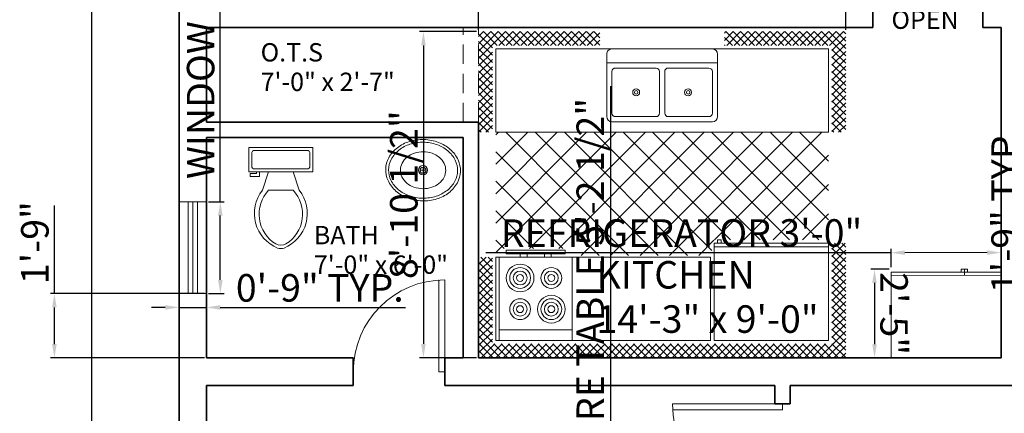
# Model space of a CAD drawing. Units: inches. Extents: x 1885 to 4781, y 1153 to 4395.
# Tile 2 of 7: x 2309 to 2631, y 1657 to 1786. Entities that reach past the tile are written whole.
import ezdxf

# ---------------------------------------------------------------- set-up
doc = ezdxf.new("R2010")
doc.units = ezdxf.units.IN
doc.linetypes.add('HIDDEN', pattern=[9.525, 6.35, -3.175])
doc.layers.add('A-ANNO-DIMS', color=5, linetype='Continuous', lineweight=18)
doc.layers.add('A-WALL', color=7, linetype='Continuous', lineweight=35)
for name, color, linetype, lineweight, true_color in [('A-ANNO-TEXT', 244, 'Continuous', 18, 0x991b1e), ('A-AREA-IDEN', 244, 'Continuous', 18, 0x991b1e), ('A-DOOR', 11, 'Continuous', 18, 0xf27172), ('A-EQPM', 11, 'Continuous', 18, 0xf27172), ('A-FLOR-FIXT', 11, 'Continuous', 18, 0xf27172), ('A-GLAZ', 152, 'Continuous', 18, 0x2776bb), ('A-WALL-HIDN', 11, 'HIDDEN', 18, 0xf27172)]:
    doc.layers.add(name, color=color, linetype=linetype, lineweight=lineweight, true_color=true_color)
doc.styles.get("Standard").update_dxf_attribs({"font": 'arial.ttf'})
doc.dimstyles.new('ISO-25', dxfattribs={"dimtxt": 9, "dimasz": 4.5, "dimexe": 1.25, "dimexo": 0.625, "dimtad": 1, "dimdec": 0, "dimlunit": 3, "dimtxsty": 'Standard', "dimcen": 2.5, "dimadec": 0, "dimazin": 0, "dimtfac": 1, "dimtdec": 0, "dimtmove": 0, "dimatfit": 3, "dimfxl": 1, "dimarcsym": 0})

# ---------------------------------------------------------------- blocks, each defined once
blk = doc.blocks.new('Kitchen Layout - 7 x 8 ft')
for p, q in [((-5, 81.32), (2.68, 89)), ((-5, 83.44), (0.56, 89)), ((-5, 85.56), (-1.56, 89)), ((-5, 87.68), (-3.68, 89)), ((-1, 84.97), (-5, 88.97)), ((1.09, 85), (-2.91, 89)), ((3.21, 85), (-0.79, 89)), ((0.81, 85), (4.81, 89)), ((5.34, 85), (1.34, 89)), ((2.93, 85), (6.93, 89)), ((7.46, 85), (3.46, 89)), ((5.05, 85), (9.05, 89)), ((9.58, 85), (5.58, 89)), ((7.17, 85), (11.17, 89)), ((11.7, 85), (7.7, 89)), ((9.29, 85), (13.29, 89)), ((13.82, 85), (9.82, 89)), ((11.41, 85), (15.41, 89)), ((15.94, 85), (11.94, 89)), ((13.53, 85), (17.53, 89)), ((18.06, 85), (14.06, 89)), ((15.65, 85), (19.65, 89)), ((20.18, 85), (16.18, 89)), ((17.78, 85), (21.78, 89)), ((22.31, 85), (18.31, 89)), ((19.9, 85), (23.9, 89)), ((24.43, 85), (20.43, 89)), ((22.02, 85), (26.02, 89)), ((26.55, 85), (22.55, 89)), ((24.14, 85), (28.14, 89)), ((28.67, 85), (24.67, 89)), ((26.26, 85), (30.26, 89)), ((30.79, 85), (26.79, 89)), ((28.38, 85), (32.38, 89)), ((32.91, 85), (28.91, 89)), ((30.5, 85), (34.5, 89)), ((35.03, 85), (31.03, 89)), ((32.63, 85), (36.63, 89)), ((37.16, 85), (33.16, 89)), ((34.75, 85), (38.75, 89)), ((39.28, 85), (35.28, 89)), ((36.87, 85), (40.87, 89)), ((41.4, 85), (37.4, 89)), ((38.99, 85), (42.99, 89)), ((43.52, 85), (39.52, 89)), ((41.11, 85), (45.11, 89)), ((45.64, 85), (41.64, 89)), ((43.23, 85), (47.23, 89)), ((47.76, 85), (43.76, 89)), ((45.35, 85), (49.35, 89)), ((49.88, 85), (45.88, 89)), ((47.47, 85), (51.47, 89)), ((52, 85), (48, 89)), ((49.6, 85), (53.6, 89)), ((54.13, 85), (50.13, 89)), ((51.72, 85), (55.72, 89)), ((56.25, 85), (52.25, 89)), ((53.84, 85), (57.84, 89)), ((58.37, 85), (54.37, 89)), ((55.96, 85), (59.96, 89)), ((60.49, 85), (56.49, 89)), ((58.08, 85), (62.08, 89)), ((62.61, 85), (58.61, 89)), ((60.2, 85), (64.2, 89)), ((64.73, 85), (60.73, 89)), ((62.32, 85), (66.32, 89)), ((66.85, 85), (62.85, 89)), ((64.45, 85), (68.45, 89)), ((68.97, 85), (64.97, 89)), ((66.57, 85), (70.57, 89)), ((71.1, 85), (67.1, 89)), ((68.69, 85), (72.69, 89)), ((73.22, 85), (69.22, 89)), ((70.81, 85), (74.81, 89)), ((75.34, 85), (71.34, 89)), ((72.93, 85), (76.93, 89)), ((77.46, 85), (73.46, 89)), ((75.05, 85), (79.05, 89)), ((79.58, 85), (75.58, 89)), ((77.17, 85), (81.17, 89)), ((81.7, 85), (77.7, 89)), ((79.29, 85), (83.29, 89)), ((83.82, 85), (79.82, 89)), ((81.42, 85), (85.42, 89)), ((85.95, 85), (81.95, 89)), ((83.54, 85), (87.54, 89)), ((88.07, 85), (84.07, 89)), ((85.66, 85), (89.66, 89)), ((90.19, 85), (86.19, 89)), ((87.78, 85), (91.78, 89)), ((92.31, 85), (88.31, 89)), ((89.9, 85), (93.9, 89)), ((94.43, 85), (90.43, 89)), ((92.02, 85), (96.02, 89)), ((96.55, 85), (92.55, 89)), ((94.14, 85), (98.14, 89)), ((101, 82.67), (94.67, 89)), ((96.27, 85), (100.27, 89)), ((101, 84.79), (96.79, 89)), ((101, 86.92), (98.92, 89)), ((-1, 82.85), (-5, 86.85)), ((97, 83.61), (101, 87.61)), ((97, 81.49), (101, 85.49)), ((-1, 80.73), (-5, 84.73)), ((-5, 79.19), (-1, 83.19)), ((-1, 78.61), (-5, 82.61)), ((34, 84), (96, 84)), ((34, 60), (34, 84)), ((96, 84), (96, 60)), ((101, 80.55), (97, 84.55)), ((97, 79.37), (101, 83.37)), ((-5, 77.07), (-1, 81.07)), ((-1, 76.49), (-5, 80.49)), ((74, 81), (95, 81)), ((101, 78.43), (97, 82.43)), ((97, 77.25), (101, 81.25)), ((101, 76.31), (97, 80.31)), ((-5, 74.95), (-1, 78.95)), ((-1, 74.36), (-5, 78.36)), ((-5, 72.83), (-1, 76.83)), ((97, 75.13), (101, 79.13)), ((101, 74.19), (97, 78.19)), ((97, 73.01), (101, 77.01)), ((-1, 72.24), (-5, 76.24)), ((-5, 70.71), (-1, 74.71)), ((-1, 70.12), (-5, 74.12)), ((101, 72.07), (97, 76.07)), ((97, 70.89), (101, 74.89)), ((101, 69.95), (97, 73.95)), ((-5, 68.59), (-1, 72.59)), ((-1, 68), (-5, 72)), ((97, 68.76), (101, 72.76)), ((101, 67.82), (97, 71.82)), ((-5, 66.47), (-1, 70.47)), ((-1, 65.88), (-5, 69.88)), ((-5, 64.35), (-1, 68.35)), ((97, 66.64), (101, 70.64)), ((101, 65.7), (97, 69.7)), ((97, 64.52), (101, 68.52)), ((-1, 63.76), (-5, 67.76)), ((-5, 62.22), (-1, 66.22)), ((-1, 61.64), (-5, 65.64)), ((101, 63.58), (97, 67.58)), ((97, 62.4), (101, 66.4)), ((101, 61.46), (97, 65.46)), ((-5, 60.1), (-1, 64.1)), ((-1, 59.52), (-5, 63.52)), ((97, 60.28), (101, 64.28)), ((100.34, 60), (97, 63.34)), ((-5, 57.98), (-1, 61.98)), ((-1, 57.39), (-5, 61.39)), ((-4.86, 56), (-1, 59.86)), ((96, 60), (34, 60)), ((80, 60), (80, 59)), ((82, 59), (82, 60)), ((87, 59), (87, 60)), ((89, 60), (89, 59)), ((98.22, 60), (97, 61.22)), ((98.84, 60), (101, 62.16)), ((100.96, 60), (101, 60.04)), ((-1.73, 56), (-5, 59.27)), ((-3.85, 56), (-5, 57.15)), ((-2.74, 56), (-1, 57.74)), ((0, 57), (33, 57)), ((10.4, 24), (45.9, 59.5)), ((18.88, 24), (54.38, 59.5)), ((27.37, 24), (62.87, 59.5)), ((33.03, 55.11), (37.41, 59.5)), ((67.71, 24), (33.68, 58.04)), ((35.85, 24), (71.35, 59.5)), ((76.2, 24), (40.7, 59.5)), ((44.34, 24), (77.84, 57.5)), ((84.68, 24), (49.18, 59.5)), ((52.82, 24), (86.32, 57.5)), ((93.17, 24), (57.67, 59.5)), ((61.31, 24), (96, 58.69)), ((96, 29.65), (66.15, 59.5)), ((96, 38.14), (76.64, 57.5)), ((96, 46.63), (85.13, 57.5)), ((96, 55.11), (93.57, 57.54)), ((0, 30.57), (24.43, 55)), ((0, 39.06), (15.94, 55)), ((0, 47.54), (7.46, 55)), ((1.91, 24), (32.91, 55)), ((33.77, 24), (2.77, 55)), ((42.26, 24), (11.26, 55)), ((50.74, 24), (19.74, 55)), ((59.23, 24), (28.23, 55)), ((31, 55), (31, 56)), ((32, 55), (31, 55)), ((32, 56), (32, 55)), ((25.29, 24), (0, 49.29)), ((69.79, 24), (96, 50.21)), ((16.8, 24), (0, 40.8)), ((78.28, 24), (96, 41.72)), ((8.32, 24), (0, 32.32)), ((86.76, 24), (96, 33.24)), ((-5, 21.92), (-2.92, 24)), ((-5, 19.8), (-1, 23.8)), ((-1, 19.21), (-5, 23.21)), ((-1, 21.33), (-3.67, 24)), ((-1, 23.45), (-1.55, 24)), ((0, 24), (96, 24)), ((0, 0), (0, 24)), ((95.25, 24), (96, 24.75)), ((96, 24), (96, 0)), ((97, 22.1), (98.9, 24)), ((97, 19.97), (101, 23.97)), ((101, 19.03), (97, 23.03)), ((101, 21.16), (98.16, 24)), ((101, 23.28), (100.28, 24)), ((-5, 17.68), (-1, 21.68)), ((-1, 17.09), (-5, 21.09)), ((97, 17.85), (101, 21.85)), ((101, 16.91), (97, 20.91)), ((-5, 15.55), (-1, 19.55)), ((-1, 14.97), (-5, 18.97)), ((-5, 13.43), (-1, 17.43)), ((47.25, 6.5), (47.25, 18.5)), ((48.75, 18.5), (48.75, 6.5)), ((97, 15.73), (101, 19.73)), ((101, 14.79), (97, 18.79)), ((97, 13.61), (101, 17.61)), ((-1, 12.85), (-5, 16.85)), ((-5, 11.31), (-1, 15.31)), ((-1, 10.73), (-5, 14.73)), ((101, 12.67), (97, 16.67)), ((97, 11.49), (101, 15.49)), ((101, 10.55), (97, 14.55)), ((-5, 9.19), (-1, 13.19)), ((-1, 8.6), (-5, 12.6)), ((97, 9.37), (101, 13.37)), ((101, 8.43), (97, 12.43)), ((-5, 7.07), (-1, 11.07)), ((-1, 6.48), (-5, 10.48)), ((-5, 4.95), (-1, 8.95)), ((97, 7.25), (101, 11.25)), ((101, 6.31), (97, 10.31)), ((97, 5.12), (101, 9.12)), ((-1, 4.36), (-5, 8.36)), ((-5, 2.83), (-1, 6.83)), ((-1, 2.24), (-5, 6.24)), ((101, 4.18), (97, 8.18)), ((97, 3), (101, 7)), ((101, 2.06), (97, 6.06)), ((-5, 0.71), (-1, 4.71)), ((-1, 0.12), (-5, 4.12)), ((64, 4), (32, 4)), ((97, 0.88), (101, 4.88)), ((101, -0.06), (97, 3.94)), ((-5, -1.42), (-1, 2.58)), ((2, -5), (-5, 2)), ((-5, -3.54), (-1, 0.46)), ((96, 0), (0, 0)), ((93.24, -5), (101, 2.76)), ((95.36, -5), (101, 0.64)), ((101, -2.18), (97, 1.82)), ((-0.12, -5), (-5, -0.12)), ((-2.25, -5), (-5, -2.25)), ((-4.34, -5), (-0.34, -1)), ((-2.22, -5), (1.78, -1)), ((-0.1, -5), (3.9, -1)), ((4.12, -5), (0.12, -1)), ((2.02, -5), (6.02, -1)), ((6.24, -5), (2.24, -1)), ((4.14, -5), (8.14, -1)), ((8.36, -5), (4.36, -1)), ((6.27, -5), (10.27, -1)), ((10.48, -5), (6.48, -1)), ((8.39, -5), (12.39, -1)), ((12.6, -5), (8.6, -1)), ((10.51, -5), (14.51, -1)), ((14.73, -5), (10.73, -1)), ((12.63, -5), (16.63, -1)), ((16.85, -5), (12.85, -1)), ((14.75, -5), (18.75, -1)), ((18.97, -5), (14.97, -1)), ((16.87, -5), (20.87, -1)), ((21.09, -5), (17.09, -1)), ((18.99, -5), (22.99, -1)), ((23.21, -5), (19.21, -1)), ((21.11, -5), (25.11, -1)), ((25.33, -5), (21.33, -1)), ((23.24, -5), (27.24, -1)), ((27.45, -5), (23.45, -1)), ((25.36, -5), (29.36, -1)), ((29.57, -5), (25.57, -1)), ((27.48, -5), (30, -2.48)), ((30, -3.3), (27.7, -1)), ((30, -1.18), (29.82, -1)), ((66, -2.54), (67.54, -1)), ((66, -4.66), (69.66, -1)), ((69.88, -5), (66, -1.12)), ((67.78, -5), (71.78, -1)), ((72, -5), (68, -1)), ((69.9, -5), (73.9, -1)), ((74.12, -5), (70.12, -1)), ((72.03, -5), (76.03, -1)), ((76.24, -5), (72.24, -1)), ((74.15, -5), (78.15, -1)), ((78.36, -5), (74.36, -1)), ((76.27, -5), (80.27, -1)), ((80.49, -5), (76.49, -1)), ((78.39, -5), (82.39, -1)), ((82.61, -5), (78.61, -1)), ((80.51, -5), (84.51, -1)), ((84.73, -5), (80.73, -1)), ((82.63, -5), (86.63, -1)), ((86.85, -5), (82.85, -1)), ((84.75, -5), (88.75, -1)), ((88.97, -5), (84.97, -1)), ((86.88, -5), (90.88, -1)), ((91.09, -5), (87.09, -1)), ((89, -5), (93, -1)), ((93.21, -5), (89.21, -1)), ((91.12, -5), (95.12, -1)), ((95.34, -5), (91.34, -1)), ((97.46, -5), (93.46, -1)), ((99.58, -5), (95.58, -1)), ((101, -4.3), (97, -0.3)), ((97.48, -5), (101, -1.48)), ((-4.37, -5), (-5, -4.37)), ((29.6, -5), (30, -4.6)), ((67.76, -5), (66, -3.24)), ((99.6, -5), (101, -3.6))]:
    blk.add_line(p, q)
for points in [[(0, 56), (0, 84), (33, 84), (33, 56)], [(74, 60), (74, 84), (95, 84), (95, 60)], [(76, 58), (76, 59), (93, 59), (93, 58)]]:
    blk.add_lwpolyline(points, close=True)
for points in [[(33.5, 21), (62.5, 21)], [(32, 1.5), (32, 19.5)], [(33.5, 6.5), (33.5, 18.5)], [(34.5, 19.5), (46.25, 19.5)], [(49.75, 19.5), (61.5, 19.5)], [(62.5, 18.5), (62.5, 6.5)], [(64, 19.5), (64, 1.5)], [(46.25, 5.5), (34.5, 5.5)], [(61.5, 5.5), (49.75, 5.5)], [(62.5, 0), (33.5, 0)]]:
    blk.add_lwpolyline(points)
for centre, radius in [((80, 75), 4), ((80, 75), 3), ((80, 75), 2), ((89, 75), 3), ((89, 75), 2), ((80, 75), 1), ((89, 75), 1), ((80, 66), 3), ((89, 66), 4), ((89, 66), 3), ((80, 66), 2), ((80, 66), 1), ((89, 66), 2), ((89, 66), 1), ((40.5, 12.5), 1), ((40.5, 12.5), 0.5), ((55.5, 12.5), 1), ((55.5, 12.5), 0.5)]:
    blk.add_circle(centre, radius)
for centre, radius, start, end in [((33.5, 19.5), 1.5, 90, 180), ((62.5, 19.5), 1.5, 0, 90), ((34.5, 18.5), 1, 90, 180), ((46.25, 18.5), 1, 0, 90), ((49.75, 18.5), 1, 90, 180), ((61.5, 18.5), 1, 0, 90), ((34.5, 6.5), 1, 180, 270), ((46.25, 6.5), 1, 270, 0), ((49.75, 6.5), 1, 180, 270), ((61.5, 6.5), 1, 270, 0), ((33.5, 1.5), 1.5, 180, 270), ((62.5, 1.5), 1.5, 270, 0)]:
    blk.add_arc(centre, radius, start, end)
blk = doc.blocks.new('Refrigerator-2 door - 36 in top')
for p, q in [((0, -26.999999), (36, -26.999999)), ((11, -27.999999), (11, -28.999999)), ((12, -26.999999), (12, -28.999999)), ((13, -28.999999), (13, -27.999999)), ((11, -28.999999), (13, -28.999999))]:
    blk.add_line(p, q)
blk.add_lwpolyline([(0, -27.999999), (0, 0), (36, 0), (36, -27.999999)], close=True)
blk = doc.blocks.new('Toilet - top')
for p, q in [((9.5, -6), (9.5, -2)), ((-10, -8.5), (-8, -8.5)), ((-10, -9.5), (-10, -8.5)), ((-7, -9.5), (-10, -9.5)), ((-8, -8.5), (-8, -8)), ((-7, -8), (-7, -9.5)), ((-4, -8), (-6, -14)), ((4, -8), (6, -14)), ((4, -14), (-4, -14))]:
    blk.add_line(p, q)
blk.add_lwpolyline([(10.5, -8), (10.5, 0), (-10.5, 0), (-10.5, -8)], close=True)
for points in [[(-9.5, -2), (-9.5, -6)], [(8.5, -1), (-8.5, -1)], [(-8.5, -7), (8.5, -7)]]:
    blk.add_lwpolyline(points)
for centre, radius, start, end in [((-8.62, -1.88), 0.884, 81.8699, 188.1301), ((8.62, -1.88), 0.884, 351.8699, 98.1301), ((-8.62, -6.12), 0.884, 171.8699, 278.1301), ((8.62, -6.12), 0.884, 261.8699, 8.1301), ((3.52, -21.58), 12.17, 141.4691, 247.9714), ((4.2, -21.82), 11.33, 136.3677, 238.9468), ((-3.52, -21.58), 12.17, 292.0284, 38.5307), ((-4.2, -21.82), 11.33, 301.053, 43.6321), ((0, -27.88), 4, 245.7318, 294.2682), ((0, -29), 4, 254.8605, 285.1395)]:
    blk.add_arc(centre, radius, start, end)
blk = doc.blocks.new('Sink - Oval top')
for p, q in [((-1, 0), (1, 0)), ((0, 1), (0, -1))]:
    blk.add_line(p, q)
for points in [[(-12.23, 0.39, 0.117634), (-11.46, -3.36, 0.104469), (-8.88, -6.8, 0.090016), (-5.08, -9.07, 0.08192), (-0.32, -10.02, 0.08192), (4.49, -9.38, 0.090016), (8.42, -7.36, 0.104469), (11.22, -4.09, 0.117634), (12.23, -0.39, 0.117634), (11.46, 3.36, 0.104469), (8.88, 6.8, 0.090016), (5.08, 9.07, 0.08192), (0.32, 10.02, 0.08192), (-4.49, 9.38, 0.090016), (-8.42, 7.36, 0.104469), (-11.22, 4.09, 0.117634)], [(-11.29, 0.16, 0.118622), (-10.52, -3.25, 0.104678), (-8.07, -6.36, 0.089562), (-4.54, -8.37, 0.081185), (-0.13, -9.15, 0.081185), (4.3, -8.49, 0.089562), (7.89, -6.58, 0.104678), (10.42, -3.55, 0.118622), (11.29, -0.16, 0.118622), (10.52, 3.25, 0.104678), (8.07, 6.36, 0.089562), (4.54, 8.37, 0.081185), (0.13, 9.15, 0.081185), (-4.3, 8.49, 0.089562), (-7.89, 6.58, 0.104678), (-10.42, 3.55, 0.118622)], [(-7.42, 0.08, 0.118283), (-6.91, -2.17, 0.104607), (-5.29, -4.21, 0.089718), (-2.97, -5.53, 0.081436), (-0.07, -6.04, 0.081436), (2.84, -5.59, 0.089718), (5.2, -4.33, 0.104607), (6.86, -2.32, 0.118283), (7.42, -0.08, 0.118283), (6.91, 2.17, 0.104607), (5.29, 4.21, 0.089718), (2.97, 5.53, 0.081436), (0.07, 6.04, 0.081436), (-2.84, 5.59, 0.089718), (-5.2, 4.33, 0.104607), (-6.86, 2.32, 0.118283)]]:
    blk.add_lwpolyline(points, format="xyb", close=True)
for radius in [1.5, 1]:
    blk.add_circle((0, 0), radius)
blk = doc.blocks.new('*D26')
at = {"layer": 'A-ANNO-DIMS', "color": 0, "lineweight": -2, "transparency": 16777216}
for p, q in [((2360.28, 2222.42), (2331.02, 2222.42)), ((2332.27, 2217.92), (2332.27, 1493.92)), ((2360.28, 1489.42), (2331.02, 1489.42))]:
    blk.add_line(p, q, dxfattribs=at)
at = {"layer": 'A-ANNO-DIMS', "color": 0, "transparency": 16777216}
for points in [[(2331.52, 2217.92), (2333.02, 2217.92), (2332.27, 2222.42)], [(2331.52, 1493.92), (2333.02, 1493.92), (2332.27, 1489.42)]]:
    blk.add_solid(points, dxfattribs=at)
at = {"layer": 'Defpoints', "color": 0, "transparency": 16777216}
for p in [(2360.91, 2222.42), (2332.27, 1489.42), (2360.91, 1489.42)]:
    blk.add_point(p, dxfattribs=at)
at = {"layer": 'A-ANNO-DIMS', "color": 0, "transparency": 16777216, "insert": (2327.04, 1855.92), "char_height": 9, "attachment_point": 5, "rotation": 90}
blk.add_mtext('61\'-1"', dxfattribs=at)
blk = doc.blocks.new('WIN-30IN')
for p, q in [((0, 0), (0, 30)), ((0, 30), (9, 30)), ((3, 0), (3, 30)), ((4.5, 0), (4.5, 30)), ((6, 0), (6, 30)), ((9, 30), (9, 0)), ((9, 0), (0, 0))]:
    blk.add_line(p, q)
blk = doc.blocks.new('DOOR-SWING-30IN')
for p, q in [((0, 2), (30, 2)), ((30, 0), (30, 2)), ((0, 0), (30, 0))]:
    blk.add_line(p, q)
blk.add_arc((30, 0), 30, 90, 180)
blk = doc.blocks.new('DOOR-SWING-36IN')
for p, q in [((0, 36), (0, 0)), ((2, 36), (2, 0)), ((0, 0), (2, 0))]:
    blk.add_line(p, q)
blk.add_arc((0, 0), 36, 0, 90)
blk = doc.blocks.new('*D47')
at = {"layer": 'A-ANNO-DIMS', "color": 0, "lineweight": -2, "transparency": 16777216}
for p, q in [((2374.41, 1726.42), (2374.41, 1846.06)), ((2370.53, 1726.42), (2375.66, 1726.42)), ((2374.41, 1700.92), (2374.41, 1721.92)), ((2370.53, 1696.42), (2375.66, 1696.42))]:
    blk.add_line(p, q, dxfattribs=at)
at = {"layer": 'A-ANNO-DIMS', "color": 0, "transparency": 16777216}
for points in [[(2373.66, 1721.92), (2375.16, 1721.92), (2374.41, 1726.42)], [(2373.66, 1700.92), (2375.16, 1700.92), (2374.41, 1696.42)]]:
    blk.add_solid(points, dxfattribs=at)
at = {"layer": 'Defpoints', "color": 0, "transparency": 16777216}
for p in [(2369.91, 1726.42), (2374.41, 1726.42), (2369.91, 1696.42)]:
    blk.add_point(p, dxfattribs=at)
at = {"layer": 'A-ANNO-DIMS', "color": 0, "transparency": 16777216, "insert": (2369.13, 1788.49), "char_height": 9, "attachment_point": 5, "rotation": 90}
blk.add_mtext('WINDOW 2\'-6" TYP.', dxfattribs=at)
blk = doc.blocks.new('*D48')
at = {"layer": 'A-ANNO-DIMS', "color": 0, "lineweight": -2, "transparency": 16777216}
for p, q in [((2360.91, 1695.8), (2360.91, 1690.67)), ((2369.91, 1695.8), (2369.91, 1690.67)), ((2356.41, 1691.92), (2351.91, 1691.92)), ((2360.91, 1691.92), (2369.91, 1691.92)), ((2374.41, 1691.92), (2435.02, 1691.92))]:
    blk.add_line(p, q, dxfattribs=at)
at = {"layer": 'A-ANNO-DIMS', "color": 0, "transparency": 16777216}
for points in [[(2356.41, 1692.67), (2356.41, 1691.17), (2360.91, 1691.92)], [(2374.41, 1692.67), (2374.41, 1691.17), (2369.91, 1691.92)]]:
    blk.add_solid(points, dxfattribs=at)
at = {"layer": 'Defpoints', "color": 0, "transparency": 16777216}
for p in [(2360.91, 1696.42), (2369.91, 1696.42), (2369.91, 1691.92)]:
    blk.add_point(p, dxfattribs=at)
at = {"layer": 'A-ANNO-DIMS', "color": 0, "transparency": 16777216, "insert": (2406.96, 1697.14), "char_height": 9, "attachment_point": 5}
blk.add_mtext('0\'-9" TYP.', dxfattribs=at)
blk = doc.blocks.new('*D56')
at = {"layer": 'A-ANNO-DIMS', "color": 0, "lineweight": -2, "transparency": 16777216}
for p, q in [((2637.61, 1691.92), (2637.61, 1751.68)), ((2643.28, 1691.92), (2636.36, 1691.92)), ((2637.61, 1675.42), (2637.61, 1687.42)), ((2643.28, 1670.92), (2636.36, 1670.92))]:
    blk.add_line(p, q, dxfattribs=at)
at = {"layer": 'A-ANNO-DIMS', "color": 0, "transparency": 16777216}
for points in [[(2636.86, 1687.42), (2638.36, 1687.42), (2637.61, 1691.92)], [(2636.86, 1675.42), (2638.36, 1675.42), (2637.61, 1670.92)]]:
    blk.add_solid(points, dxfattribs=at)
at = {"layer": 'Defpoints', "color": 0, "transparency": 16777216}
for p in [(2637.61, 1691.92), (2643.91, 1691.92), (2643.91, 1670.92)]:
    blk.add_point(p, dxfattribs=at)
at = {"layer": 'A-ANNO-DIMS', "color": 0, "transparency": 16777216, "insert": (2632.39, 1724.05), "char_height": 9, "attachment_point": 5, "rotation": 90}
blk.add_mtext('1\'-9" TYP.', dxfattribs=at)
blk = doc.blocks.new('*D61')
at = {"layer": 'A-ANNO-DIMS', "color": 0, "lineweight": -2, "transparency": 16777216}
for p, q in [((2502.19, 1613.69), (2502.19, 1764.21)), ((2493.47, 1613.69), (2503.44, 1613.69)), ((2502.19, 1555.92), (2502.19, 1609.19)), ((2493.47, 1551.42), (2503.44, 1551.42))]:
    blk.add_line(p, q, dxfattribs=at)
at = {"layer": 'A-ANNO-DIMS', "color": 0, "transparency": 16777216}
for points in [[(2501.44, 1609.19), (2502.94, 1609.19), (2502.19, 1613.69)], [(2501.44, 1555.92), (2502.94, 1555.92), (2502.19, 1551.42)]]:
    blk.add_solid(points, dxfattribs=at)
at = {"layer": 'Defpoints', "color": 0, "transparency": 16777216}
for p in [(2492.84, 1613.69), (2502.19, 1613.69), (2492.84, 1551.42)]:
    blk.add_point(p, dxfattribs=at)
at = {"layer": 'A-ANNO-DIMS', "color": 0, "transparency": 16777216, "insert": (2496.63, 1691.2), "char_height": 9, "attachment_point": 5, "rotation": 90}
blk.add_mtext('SQUARE TABLE 5\'-2 1/2"', dxfattribs=at)
blk = doc.blocks.new('*D67')
at = {"layer": 'A-ANNO-DIMS', "color": 0, "lineweight": -2, "transparency": 16777216}
for p, q in [((2458.91, 1782.66), (2458.91, 1801.3)), ((2579.06, 1782.66), (2579.06, 1801.3)), ((2574.56, 1800.05), (2463.41, 1800.05))]:
    blk.add_line(p, q, dxfattribs=at)
at = {"layer": 'A-ANNO-DIMS', "color": 0, "transparency": 16777216}
for points in [[(2463.41, 1800.8), (2463.41, 1799.3), (2458.91, 1800.05)], [(2574.56, 1800.8), (2574.56, 1799.3), (2579.06, 1800.05)]]:
    blk.add_solid(points, dxfattribs=at)
at = {"layer": 'Defpoints', "color": 0, "transparency": 16777216}
for p in [(2458.91, 1800.05), (2458.91, 1782.03), (2579.06, 1782.03)]:
    blk.add_point(p, dxfattribs=at)
at = {"layer": 'A-ANNO-DIMS', "color": 0, "transparency": 16777216, "insert": (2518.99, 1805.34), "char_height": 9, "attachment_point": 5}
blk.add_mtext('CASEWORK 10\'-0"', dxfattribs=at)
blk = doc.blocks.new('*D68')
at = {"layer": 'A-ANNO-DIMS', "color": 0, "lineweight": -2, "transparency": 16777216}
for p, q in [((2458.28, 1782.03), (2439.63, 1782.03)), ((2440.88, 1777.53), (2440.88, 1679.98)), ((2458.28, 1675.48), (2439.63, 1675.48))]:
    blk.add_line(p, q, dxfattribs=at)
at = {"layer": 'A-ANNO-DIMS', "color": 0, "transparency": 16777216}
for points in [[(2440.13, 1777.53), (2441.63, 1777.53), (2440.88, 1782.03)], [(2440.13, 1679.98), (2441.63, 1679.98), (2440.88, 1675.48)]]:
    blk.add_solid(points, dxfattribs=at)
at = {"layer": 'Defpoints', "color": 0, "transparency": 16777216}
for p in [(2458.91, 1782.03), (2440.88, 1675.48), (2458.91, 1675.48)]:
    blk.add_point(p, dxfattribs=at)
at = {"layer": 'A-ANNO-DIMS', "color": 0, "transparency": 16777216, "insert": (2435.61, 1728.75), "char_height": 9, "attachment_point": 5, "rotation": 90}
blk.add_mtext('8\'-10 1/2"', dxfattribs=at)
blk = doc.blocks.new('*D69')
at = {"layer": 'A-ANNO-DIMS', "color": 0, "lineweight": -2, "transparency": 16777216}
for p, q in [((2593.89, 1705.02), (2593.89, 1711.05)), ((2629.89, 1705.05), (2629.89, 1711.07)), ((2593.89, 1709.8), (2461.3, 1709.72)), ((2625.39, 1709.82), (2598.39, 1709.8))]:
    blk.add_line(p, q, dxfattribs=at)
at = {"layer": 'A-ANNO-DIMS', "color": 0, "transparency": 16777216}
for points in [[(2598.39, 1710.55), (2598.39, 1709.05), (2593.89, 1709.8)], [(2625.39, 1710.57), (2625.39, 1709.07), (2629.89, 1709.82)]]:
    blk.add_solid(points, dxfattribs=at)
at = {"layer": 'Defpoints', "color": 0, "transparency": 16777216}
for p in [(2593.89, 1709.8), (2593.89, 1704.4), (2629.89, 1704.42)]:
    blk.add_point(p, dxfattribs=at)
at = {"layer": 'A-ANNO-DIMS', "color": 0, "transparency": 16777216, "insert": (2525.34, 1715.04), "char_height": 9, "attachment_point": 5, "rotation": 0.0343}
blk.add_mtext('REFRIGERATOR 3\'-0"', dxfattribs=at)
blk = doc.blocks.new('*D70')
at = {"layer": 'A-ANNO-DIMS', "color": 0, "lineweight": -2, "transparency": 16777216}
for p, q in [((2593.27, 1704.4), (2587.24, 1704.4)), ((2588.49, 1699.9), (2588.5, 1679.9)), ((2593.28, 1675.4), (2587.26, 1675.4))]:
    blk.add_line(p, q, dxfattribs=at)
at = {"layer": 'A-ANNO-DIMS', "color": 0, "transparency": 16777216}
for points in [[(2589.24, 1699.9), (2587.74, 1699.9), (2588.49, 1704.4)], [(2589.25, 1679.9), (2587.75, 1679.9), (2588.51, 1675.4)]]:
    blk.add_solid(points, dxfattribs=at)
at = {"layer": 'Defpoints', "color": 0, "transparency": 16777216}
for p in [(2593.89, 1704.4), (2588.51, 1675.4), (2593.91, 1675.4)]:
    blk.add_point(p, dxfattribs=at)
at = {"layer": 'A-ANNO-DIMS', "color": 0, "transparency": 16777216, "insert": (2593.72, 1689.9), "char_height": 9, "attachment_point": 5, "rotation": 270.0343}
blk.add_mtext('2\'-5"', dxfattribs=at)
blk = doc.blocks.new('*D84')
at = {"layer": 'A-ANNO-DIMS', "color": 0, "lineweight": -2, "transparency": 16777216}
for p, q in [((2320.11, 1696.42), (2320.11, 1725.25)), ((2369.28, 1696.42), (2318.86, 1696.42)), ((2320.11, 1679.92), (2320.11, 1691.92)), ((2369.28, 1675.42), (2318.86, 1675.42))]:
    blk.add_line(p, q, dxfattribs=at)
at = {"layer": 'A-ANNO-DIMS', "color": 0, "transparency": 16777216}
for points in [[(2319.36, 1691.92), (2320.86, 1691.92), (2320.11, 1696.42)], [(2319.36, 1679.92), (2320.86, 1679.92), (2320.11, 1675.42)]]:
    blk.add_solid(points, dxfattribs=at)
at = {"layer": 'Defpoints', "color": 0, "transparency": 16777216}
for p in [(2320.11, 1696.42), (2369.91, 1696.42), (2369.91, 1675.42)]:
    blk.add_point(p, dxfattribs=at)
at = {"layer": 'A-ANNO-DIMS', "color": 0, "transparency": 16777216, "insert": (2314.89, 1713.08), "char_height": 9, "attachment_point": 5, "rotation": 90}
blk.add_mtext('1\'-9"', dxfattribs=at)
blk = doc.blocks.new('*D91')
at = {"layer": 'A-ANNO-DIMS', "color": 0, "lineweight": -2, "transparency": 16777216}
for p, q in [((2634.91, 1674.8), (2634.91, 1447.37)), ((2643.91, 1674.8), (2643.91, 1447.37)), ((2630.41, 1448.62), (2625.91, 1448.62)), ((2634.91, 1448.62), (2643.91, 1448.62)), ((2648.41, 1448.62), (2678.08, 1448.62))]:
    blk.add_line(p, q, dxfattribs=at)
at = {"layer": 'A-ANNO-DIMS', "color": 0, "transparency": 16777216}
for points in [[(2630.41, 1449.37), (2630.41, 1447.87), (2634.91, 1448.62)], [(2648.41, 1449.37), (2648.41, 1447.87), (2643.91, 1448.62)]]:
    blk.add_solid(points, dxfattribs=at)
at = {"layer": 'Defpoints', "color": 0, "transparency": 16777216}
for p in [(2634.91, 1675.42), (2643.91, 1675.42), (2643.91, 1448.62)]:
    blk.add_point(p, dxfattribs=at)
at = {"layer": 'A-ANNO-DIMS', "color": 0, "transparency": 16777216, "insert": (2665.49, 1453.84), "char_height": 9, "attachment_point": 5}
blk.add_mtext('0\'-9"', dxfattribs=at)

msp = doc.modelspace()

# ---------------------------------------------------------------- linework, layer by layer
at = {"layer": 'A-WALL'}
for p, q in [((2360.91, 2222.42), (2360.91, 1489.42)), ((2587.91, 1788.42), (2587.91, 1783.42)), ((2623.91, 1788.42), (2623.91, 1783.42)), ((2369.91, 1783.42), (2587.91, 1783.42)), ((2369.91, 1783.42), (2369.91, 1752.42)), ((2623.91, 1783.42), (2629.91, 1783.42)), ((2629.91, 1783.42), (2629.91, 1675.42)), ((2369.91, 1752.42), (2458.91, 1752.42)), ((2458.91, 1752.42), (2458.91, 1675.42)), ((2369.91, 1747.42), (2453.91, 1747.42)), ((2369.91, 1747.42), (2369.91, 1675.42)), ((2453.91, 1747.42), (2453.91, 1675.42)), ((2369.91, 1675.42), (2417.91, 1675.42)), ((2417.91, 1675.42), (2417.91, 1666.42)), ((2447.91, 1675.42), (2453.91, 1675.42)), ((2447.91, 1675.42), (2447.91, 1666.42)), ((2458.91, 1675.42), (2629.91, 1675.42)), ((2369.91, 1666.42), (2417.91, 1666.42)), ((2369.91, 1666.42), (2369.91, 1498.42)), ((2447.91, 1666.42), (2555.91, 1666.42)), ((2555.91, 1666.42), (2555.91, 1660.42)), ((2560.91, 1666.42), (2560.91, 1660.42)), ((2560.91, 1666.42), (2643.91, 1666.42)), ((2555.91, 1660.42), (2560.91, 1660.42))]:
    msp.add_line(p, q, dxfattribs=at)
at = {"layer": 'A-WALL-HIDN'}
for p, q in [((2453.87, 1752.42), (2453.87, 1783.42)), ((2458.91, 1752.42), (2458.91, 1783.42))]:
    msp.add_line(p, q, dxfattribs=at)

# ---------------------------------------------------------------- block references
at = {"layer": 'A-DOOR', "extrusion": (0, 0, -1), "zscale": -1}
for name, p, rotation in [('DOOR-SWING-30IN', (-2447.91, 1700.92), 270.0000000000006), ('DOOR-SWING-36IN', (-2558.41, 1660.42), 269.9999999999985)]:
    msp.add_blockref(name, p, dxfattribs=dict(at, rotation=rotation))
at = {"layer": 'A-EQPM', "xscale": 1.133540199796827, "yscale": 1.133540199796827, "zscale": 1.133540199796827, "rotation": 180}
msp.add_blockref('Kitchen Layout - 7 x 8 ft', (2573.4, 1776.36), dxfattribs=at)
at = {"layer": 'A-EQPM', "rotation": 180.0343128560528}
msp.add_blockref('Refrigerator-2 door - 36 in top', (2629.91, 1675.42), dxfattribs=at)
at = {"layer": 'A-FLOR-FIXT'}
for name, p in [('Sink - Oval top', (2440.76, 1736.75)), ('Toilet - top', (2394.21, 1744.18))]:
    msp.add_blockref(name, p, dxfattribs=at)
at = {"layer": 'A-GLAZ'}
msp.add_blockref('WIN-30IN', (2360.91, 1696.42), dxfattribs=at)

# ---------------------------------------------------------------- texts
at = {"layer": 'A-ANNO-TEXT'}
msp.add_text('OPEN', height=6, dxfattribs=at).set_placement((2594.03, 1782.93))
at = {"layer": 'A-AREA-IDEN'}
for s, height, p in [('O.T.S', 6, (2387.6, 1772.27)), ('7\'-0" x 2\'-7"', 6, (2387.6, 1762.63)), ('BATH', 6, (2405.03, 1712.53)), ('7\'-0" x 6\'-0"', 6, (2405.03, 1702.89)), ('KITCHEN', 9, (2497.52, 1698.07)), ('14\'-3" x 9\'-0"', 9, (2497.52, 1683.61))]:
    msp.add_text(s, height=height, dxfattribs=at).set_placement(p)

# ---------------------------------------------------------------- dimensions: what is measured, and where the dimension line sits
at = {"layer": 'A-ANNO-DIMS'}
for base, p1, p2, angle, override, picture, middle in [((2332.27, 1489.42), (2360.91, 2222.42), (2360.91, 1489.42), 90, {"dimclrd": 0, "dimclre": 0, "dimclrt": 0}, '*D26', (2327.04, 1855.92)), ((2440.8842, 1675.4785), (2458.9075, 1782.0313), (2458.9075, 1675.4785), 270, {"dimdec": 1, "dimlfac": 1, "dimrnd": 0, "dimzin": 1, "dimdsep": 46, "dimlunit": 4, "dimfrac": 2}, '*D68', (2435.6057, 1728.7549)), ((2320.11, 1696.42), (2369.91, 1675.42), (2369.91, 1696.42), 90, {"dimdec": 1, "dimlfac": 1, "dimrnd": 0, "dimzin": 1, "dimdsep": 46, "dimlunit": 4, "dimfrac": 2}, '*D84', (2314.89, 1713.08)), ((2588.51, 1675.4), (2593.89, 1704.4), (2593.91, 1675.4), 270.0343, {"dimdec": 1, "dimlfac": 1, "dimrnd": 0, "dimzin": 1, "dimdsep": 46, "dimlunit": 4, "dimfrac": 2}, '*D70', (2593.72, 1689.9))]:
    dim = msp.add_linear_dim(base=base, p1=p1, p2=p2, angle=angle, dimstyle='ISO-25', override=override, dxfattribs=at)
    dim.commit()
    dim.dimension.update_dxf_attribs({"geometry": picture, "text_midpoint": middle})
for base, p1, p2, angle, text, picture, middle in [((2374.41, 1726.42), (2369.91, 1696.42), (2369.91, 1726.42), 90, 'WINDOW <> TYP.', '*D47', (2369.13, 1788.49)), ((2458.9075, 1800.0546), (2579.0628, 1782.0313), (2458.9075, 1782.0313), 180, 'CASEWORK <>', '*D67', (2518.9851, 1805.3361)), ((2502.19, 1613.69), (2492.84, 1551.42), (2492.84, 1613.69), 90, 'SQUARE TABLE <>', '*D61', (2496.63, 1691.2)), ((2637.61, 1691.92), (2643.91, 1670.92), (2643.91, 1691.92), 90, '<> TYP.', '*D56', (2632.39, 1724.05)), ((2593.89, 1709.8), (2629.89, 1704.42), (2593.89, 1704.4), 180.0343, 'REFRIGERATOR <>', '*D69', (2525.34, 1715.04))]:
    dim = msp.add_linear_dim(base=base, p1=p1, p2=p2, angle=angle, text=text, dimstyle='ISO-25', override={"dimdec": 1, "dimlfac": 1, "dimrnd": 0, "dimzin": 1, "dimdsep": 46, "dimlunit": 4, "dimfrac": 2}, dxfattribs=at)
    dim.commit()
    dim.dimension.update_dxf_attribs({"geometry": picture, "text_midpoint": middle})
dim = msp.add_linear_dim(base=(2369.91, 1691.92), p1=(2360.91, 1696.42), p2=(2369.91, 1696.42), text='<> TYP.', dimstyle='ISO-25', override={"dimdec": 1, "dimlfac": 1, "dimrnd": 0, "dimzin": 1, "dimdsep": 46, "dimlunit": 4, "dimfrac": 2}, dxfattribs=at)
dim.commit()
dim.dimension.update_dxf_attribs({"geometry": '*D48', "text_midpoint": (2406.96, 1697.14)})
dim = msp.add_linear_dim(base=(2643.91, 1448.62), p1=(2634.91, 1675.42), p2=(2643.91, 1675.42), dimstyle='ISO-25', override={"dimdec": 1, "dimlfac": 1, "dimrnd": 0, "dimzin": 1, "dimdsep": 46, "dimlunit": 4, "dimfrac": 2}, dxfattribs=at)
dim.commit()
dim.dimension.update_dxf_attribs({"geometry": '*D91', "text_midpoint": (2665.49, 1453.84)})

doc.saveas('drawing.dxf')
